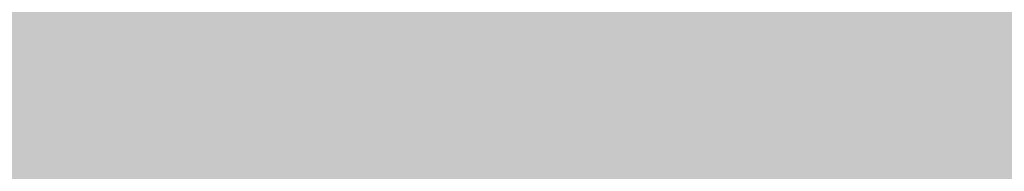
# Model space of a CAD drawing. Units: millimetres. Extents: x 0 to 2267, y 0 to 1823.
# Tile 48 of 256: x 1595.098 to 1596.855, y 1226.115 to 1226.386. Entities that reach past the tile are written whole.
import ezdxf

# ---------------------------------------------------------------- set-up
doc = ezdxf.new("R2010")
doc.units = ezdxf.units.MM
doc.header["$MEASUREMENT"] = 0
doc.layers.add('M-HATC', color=252, linetype='Continuous', lineweight=18)

msp = doc.modelspace()

# ---------------------------------------------------------------- hatches: boundary and pattern name
at = {"layer": 'M-HATC'}
h = msp.add_hatch(color=256, dxfattribs=at)
h.dxf.hatch_style = 1
h.paths.add_polyline_path([(2055.771, 1603.062), (1381.0868, 1603.062), (1381.0868, 1598.062), (2055.771, 1598.062)])
h.paths.add_polyline_path([(2055.771, 1598.062), (1381.0868, 1598.062), (1381.0868, 1593.062), (2055.771, 1593.062)])
h.paths.add_polyline_path([(2051.3074, 1536.7609), (1385.5504, 1536.7609), (1385.5504, 1526.7609), (1387.5504, 1526.7609), (1388.5366, 1525.0528), (1385.3319, 1521.2335), (1385.3319, 1521.2226), (2050.2542, 1522.7491), (2048.3212, 1525.0528), (2049.3074, 1526.7609), (2051.3074, 1526.7609)])
edge = h.paths.add_edge_path()
edge.add_arc((1847.5345, 1379.1492), 135, 222.603061, 222.890851, ccw=False)
edge.add_line((1748.1663, 1287.7656), (1683.0921, 1287.7656))
edge.add_arc((1583.7239, 1379.1492), 135, 317.109149, 317.396939, ccw=False)
edge.add_arc((1678.9686, 1290.6707), 5, 222.8909, 317.1091, ccw=False)
edge.add_arc((1774.2133, 1379.1492), 135, 222.603061, 222.890851, ccw=False)
edge.add_line((1674.8451, 1287.7656), (1609.7709, 1287.7656))
edge.add_arc((1510.4027, 1379.1492), 135, 317.109149, 317.396939, ccw=False)
edge.add_arc((1605.6474, 1290.6707), 5, 222.8909, 317.1091, ccw=False)
edge.add_arc((1700.8921, 1379.1492), 135, 222.603061, 222.890851, ccw=False)
edge.add_line((1601.5239, 1287.7656), (1536.4497, 1287.7656))
edge.add_arc((1437.0815, 1379.1492), 135, 317.109149, 317.396939, ccw=False)
edge.add_arc((1532.3262, 1290.6707), 5, 222.8909, 317.1091, ccw=False)
edge.add_arc((1627.5709, 1379.1492), 135, 222.603061, 222.890851, ccw=False)
edge.add_line((1528.2027, 1287.7656), (1505.9289, 1287.7656))
edge.add_spline(control_points=[(1505.9289, 1287.7656), (1504.2622, 1287.7656), (1504.2622, 1282.7656), (1505.9289, 1282.7656)], knot_values=[0, 0, 0, 0, 5, 5, 5, 5], degree=3, periodic=0)
edge.add_line((1505.9289, 1282.7656), (1930.9289, 1282.7656))
edge.add_spline(control_points=[(1930.9289, 1282.7656), (1932.5956, 1282.7656), (1932.5956, 1287.7656), (1930.9289, 1287.7656)], knot_values=[0, 0, 0, 0, 5, 5, 5, 5], degree=3, periodic=0)
edge.add_line((1930.9289, 1287.7656), (1903.0557, 1287.7656))
edge.add_arc((1803.6875, 1379.1492), 135, 317.109149, 317.396939, ccw=False)
edge.add_arc((1898.9322, 1290.6707), 5, 222.8909, 317.1091, ccw=False)
edge.add_arc((1994.1769, 1379.1492), 135, 222.603061, 222.890851, ccw=False)
edge.add_line((1894.8087, 1287.7656), (1829.7345, 1287.7656))
edge.add_arc((1730.3663, 1379.1492), 135, 317.109149, 317.396939, ccw=False)
edge.add_arc((1825.611, 1290.6707), 5, 222.8909, 317.1091, ccw=False)
edge.add_arc((1920.8557, 1379.1492), 135, 222.603061, 222.890851, ccw=False)
edge.add_line((1821.4875, 1287.7656), (1756.4133, 1287.7656))
edge.add_arc((1657.0451, 1379.1492), 135, 317.109149, 317.396939, ccw=False)
edge.add_arc((1752.2898, 1290.6707), 5, 222.8909, 317.1091, ccw=False)
edge = h.paths.add_edge_path()
edge.add_spline(control_points=[(1843.4289, 1227.2475), (1845.0956, 1227.2475), (1845.0956, 1232.2475), (1843.4289, 1232.2475)], knot_values=[0, 0, 0, 0, 5, 5, 5, 5], degree=3, periodic=0)
edge.add_line((1843.4289, 1232.2475), (1593.4289, 1232.2475))
edge.add_spline(control_points=[(1593.4289, 1232.2475), (1591.7622, 1232.2475), (1591.7622, 1227.2475), (1593.4289, 1227.2475)], knot_values=[0, 0, 0, 0, 5, 5, 5, 5], degree=3, periodic=0)
edge.add_line((1593.4289, 1227.2475), (1843.4289, 1227.2475))
h.paths.add_polyline_path([(1905.9289, 1127.4171), (1530.9289, 1127.4171, 0.414214), (1520.9289, 1117.4171), (1530.9289, 1117.4171), (1915.9289, 1117.4171, 0.414214)])
edge = h.paths.add_edge_path()
edge.add_arc((1397.0858, 1498.4078), 12.7299, 90.78215, 190.87871, ccw=False)
edge.add_line((1396.912, 1511.1365), (1428.0097, 1511.3488))
edge.add_line((1428.0097, 1511.3488), (1433.0097, 1511.3488))
edge.add_line((1433.0097, 1511.3488), (1434.439, 1511.3488))
edge.add_arc((1419.474, 1498.0804), 20, 41.561, 74.08211)
edge.add_line((1424.9592, 1517.3135), (1399.9351, 1517.2561))
edge.add_spline(control_points=[(1399.9307, 1517.2561), (1399.884, 1517.2131), (1399.8328, 1517.1689), (1399.7774, 1517.1236)], knot_values=[11.567499, 11.567499, 11.567499, 11.567499, 11.814249, 11.814249, 11.814249, 11.814249], degree=3, periodic=0)
edge.add_spline(control_points=[(1399.6328, 1517.0099), (1399.5831, 1516.9721), (1399.5307, 1516.9338), (1399.4759, 1516.8947)], knot_values=[11.167718, 11.167718, 11.167718, 11.167718, 11.365188, 11.365188, 11.365188, 11.365188], degree=3, periodic=0)
edge.add_spline(control_points=[(1399.3398, 1516.8001), (1399.1514, 1516.6719), (1398.9384, 1516.5377), (1398.704, 1516.3994)], knot_values=[10.376405, 10.376405, 10.376405, 10.376405, 11.00994, 11.00994, 11.00994, 11.00994], degree=3, periodic=0)
edge.add_spline(control_points=[(1398.6572, 1516.3719), (1398.5789, 1516.326), (1398.4983, 1516.2797), (1398.4155, 1516.2331)], knot_values=[10.125175, 10.125175, 10.125175, 10.125175, 10.334406, 10.334406, 10.334406, 10.334406], degree=3, periodic=0)
edge.add_spline(control_points=[(1398.2642, 1516.1487), (1398.196, 1516.1111), (1398.1263, 1516.0732), (1398.0555, 1516.0351)], knot_values=[9.832246, 9.832246, 9.832246, 9.832246, 9.999658, 9.999658, 9.999658, 9.999658], degree=3, periodic=0)
edge.add_spline(control_points=[(1397.9987, 1516.0048), (1397.7312, 1515.8621), (1397.446, 1515.7171), (1397.1466, 1515.5714)], knot_values=[9.161808, 9.161808, 9.161808, 9.161808, 9.787769, 9.787769, 9.787769, 9.787769], degree=3, periodic=0)
edge.add_spline(control_points=[(1397.1466, 1515.5714), (1396.8418, 1515.423), (1396.5222, 1515.274), (1396.1914, 1515.1262)], knot_values=[8.524455, 8.524455, 8.524455, 8.524455, 9.161808, 9.161808, 9.161808, 9.161808], degree=3, periodic=0)
edge.add_spline(control_points=[(1396.0777, 1515.0756), (1395.9854, 1515.0348), (1395.8922, 1514.994), (1395.7983, 1514.9534)], knot_values=[8.275193, 8.275193, 8.275193, 8.275193, 8.451726, 8.451726, 8.451726, 8.451726], degree=3, periodic=0)
edge.add_spline(control_points=[(1395.6018, 1514.8691), (1395.4997, 1514.8257), (1395.3968, 1514.7824), (1395.2932, 1514.7394)], knot_values=[7.962917, 7.962917, 7.962917, 7.962917, 8.152764, 8.152764, 8.152764, 8.152764], degree=3, periodic=0)
edge.add_spline(control_points=[(1395.2116, 1514.7057), (1394.8278, 1514.5475), (1394.4345, 1514.3929), (1394.0364, 1514.2442)], knot_values=[7.21254, 7.21254, 7.21254, 7.21254, 7.913148, 7.913148, 7.913148, 7.913148], degree=3, periodic=0)
edge.add_spline(control_points=[(1394.0364, 1514.2442), (1393.7076, 1514.1214), (1393.3754, 1514.0027), (1393.0427, 1513.8895)], knot_values=[6.633733, 6.633733, 6.633733, 6.633733, 7.21254, 7.21254, 7.21254, 7.21254], degree=3, periodic=0)
edge.add_spline(control_points=[(1392.8214, 1513.815), (1392.7198, 1513.7812), (1392.6181, 1513.7479), (1392.5166, 1513.7152)], knot_values=[6.328796, 6.328796, 6.328796, 6.328796, 6.505493, 6.505493, 6.505493, 6.505493], degree=3, periodic=0)
edge.add_spline(control_points=[(1392.5166, 1513.7152), (1392.3187, 1513.6515), (1392.1212, 1513.59), (1391.9244, 1513.531)], knot_values=[5.984605, 5.984605, 5.984605, 5.984605, 6.328796, 6.328796, 6.328796, 6.328796], degree=3, periodic=0)
edge.add_spline(control_points=[(1391.7915, 1513.4915), (1391.3122, 1513.3501), (1390.8384, 1513.2239), (1390.3784, 1513.1171)], knot_values=[5.066697, 5.066697, 5.066697, 5.066697, 5.907055, 5.907055, 5.907055, 5.907055], degree=3, periodic=0)
edge.add_spline(control_points=[(1390.3784, 1513.1171), (1390.1797, 1513.071), (1389.9836, 1513.0284), (1389.7907, 1512.9899)], knot_values=[4.70367, 4.70367, 4.70367, 4.70367, 5.066695, 5.066695, 5.066695, 5.066695], degree=3, periodic=0)
edge.add_spline(control_points=[(1389.422, 1512.9204), (1389.2459, 1512.8892), (1389.0729, 1512.8617), (1388.9036, 1512.8381)], knot_values=[4.130571, 4.130571, 4.130571, 4.130571, 4.469816, 4.469816, 4.469816, 4.469816], degree=3, periodic=0)
edge.add_spline(control_points=[(1388.9036, 1512.8381), (1388.591, 1512.7946), (1388.2911, 1512.7644), (1388.0071, 1512.7494)], knot_values=[3.504031, 3.504031, 3.504031, 3.504031, 4.130571, 4.130571, 4.130571, 4.130571], degree=3, periodic=0)
edge.add_spline(control_points=[(1387.9356, 1512.7459), (1387.8538, 1512.7423), (1387.7733, 1512.74), (1387.6944, 1512.739)], knot_values=[3.268866, 3.268866, 3.268866, 3.268866, 3.451164, 3.451164, 3.451164, 3.451164], degree=3, periodic=0)
edge.add_spline(control_points=[(1387.3351, 1512.7443), (1387.2076, 1512.7499), (1387.0847, 1512.7597), (1386.967, 1512.7739)], knot_values=[2.670686, 2.670686, 2.670686, 2.670686, 2.984, 2.984, 2.984, 2.984], degree=3, periodic=0)
edge.add_spline(control_points=[(1386.8327, 1512.7922), (1386.8209, 1512.7941), (1386.8092, 1512.7959), (1386.7975, 1512.7979)], knot_values=[2.516981, 2.516981, 2.516981, 2.516981, 2.549528, 2.549528, 2.549528, 2.549528], degree=3, periodic=0)
edge.add_spline(control_points=[(1386.4526, 1512.8735), (1386.4257, 1512.881), (1386.3993, 1512.889), (1386.3733, 1512.8972)], knot_values=[2.095869, 2.095869, 2.095869, 2.095869, 2.17941, 2.17941, 2.17941, 2.17941], degree=3, periodic=0)
edge.add_spline(control_points=[(1386.0691, 1513.0189), (1386.0634, 1513.0217), (1386.0577, 1513.0246), (1386.052, 1513.0275)], knot_values=[1.72453, 1.72453, 1.72453, 1.72453, 1.745933, 1.745933, 1.745933, 1.745933], degree=3, periodic=0)
edge.add_arc((1399.474, 1498.0804), 20, 131.82432, 180)
edge.add_arc((1630.3336, 1505.5484), 250.9708, 181.705176, 236.427975)
edge.add_arc((1605.3399, 1483.3044), 218.7822, 238.660829, 243.34961)
edge.add_arc((1647.0911, 1510.3592), 262.8986, 183.129836, 237.853442, ccw=False)
h.paths.add_polyline_path([(1406.5369, 1391.9644, 0.149382), (1491.5506, 1296.4418, -0.129517)], flags=17)
edge = h.paths.add_edge_path()
edge.add_arc((2037.3838, 1498.0804), 20, 0, 48.26587)
edge.add_spline(control_points=[(2050.6973, 1513.0052), (2050.6512, 1512.9847), (2050.6034, 1512.9655), (2050.5539, 1512.9477)], knot_values=[1.835652, 1.835652, 1.835652, 1.835652, 2.000781, 2.000781, 2.000781, 2.000781], degree=3, periodic=0)
edge.add_spline(control_points=[(2050.4616, 1512.9166), (2050.479, 1512.9221), (2050.4963, 1512.9277), (2050.5133, 1512.9335)], knot_values=[2.045477, 2.045477, 2.045477, 2.045477, 2.101389, 2.101389, 2.101389, 2.101389], degree=3, periodic=0)
edge.add_spline(control_points=[(2050.129, 1512.8342), (2050.1984, 1512.8473), (2050.2657, 1512.8623), (2050.3308, 1512.8792)], knot_values=[2.237629, 2.237629, 2.237629, 2.237629, 2.435841, 2.435841, 2.435841, 2.435841], degree=3, periodic=0)
edge.add_spline(control_points=[(2050.0946, 1512.8278), (2050.1061, 1512.8299), (2050.1176, 1512.832), (2050.129, 1512.8342)], knot_values=[2.435841, 2.435841, 2.435841, 2.435841, 2.468321, 2.468321, 2.468321, 2.468321], degree=3, periodic=0)
edge.add_spline(control_points=[(2049.7843, 1512.7851), (2049.8552, 1512.7922), (2049.9243, 1512.8008), (2049.9917, 1512.8109)], knot_values=[2.563852, 2.563852, 2.563852, 2.563852, 2.748541, 2.748541, 2.748541, 2.748541], degree=3, periodic=0)
edge.add_spline(control_points=[(2049.4052, 1512.7617), (2049.5364, 1512.7653), (2049.6629, 1512.773), (2049.7843, 1512.7851)], knot_values=[2.748541, 2.748541, 2.748541, 2.748541, 3.064882, 3.064882, 3.064882, 3.064882], degree=3, periodic=0)
edge.add_spline(control_points=[(2049.1698, 1512.7597), (2049.2336, 1512.7591), (2049.2965, 1512.7594), (2049.3584, 1512.7606)], knot_values=[3.102309, 3.102309, 3.102309, 3.102309, 3.2503, 3.2503, 3.2503, 3.2503], degree=3, periodic=0)
edge.add_spline(control_points=[(2048.8573, 1512.7691), (2048.9638, 1512.7638), (2049.068, 1512.7606), (2049.1698, 1512.7597)], knot_values=[3.2503, 3.2503, 3.2503, 3.2503, 3.486069, 3.486069, 3.486069, 3.486069], degree=3, periodic=0)
edge.add_spline(control_points=[(2048.6924, 1512.7789), (2048.3729, 1512.8009), (2048.0345, 1512.8411), (2047.6817, 1512.897)], knot_values=[3.606429, 3.606429, 3.606429, 3.606429, 4.2989, 4.2989, 4.2989, 4.2989], degree=3, periodic=0)
edge.add_spline(control_points=[(2047.6817, 1512.897), (2047.5458, 1512.9185), (2047.4077, 1512.9424), (2047.2678, 1512.9685)], knot_values=[4.2989, 4.2989, 4.2989, 4.2989, 4.565769, 4.565769, 4.565769, 4.565769], degree=3, periodic=0)
edge.add_spline(control_points=[(2047.2678, 1512.9685), (2047.1449, 1512.9914), (2047.0207, 1513.016), (2046.8951, 1513.0422)], knot_values=[4.565769, 4.565769, 4.565769, 4.565769, 4.799971, 4.799971, 4.799971, 4.799971], degree=3, periodic=0)
edge.add_spline(control_points=[(2046.8951, 1513.0422), (2046.5286, 1513.1188), (2046.1513, 1513.209), (2045.7676, 1513.3107)], knot_values=[4.799971, 4.799971, 4.799971, 4.799971, 5.483718, 5.483718, 5.483718, 5.483718], degree=3, periodic=0)
edge.add_spline(control_points=[(2045.7676, 1513.3107), (2045.3724, 1513.4154), (2044.9704, 1513.5322), (2044.5662, 1513.6588)], knot_values=[5.483718, 5.483718, 5.483718, 5.483718, 6.187866, 6.187866, 6.187866, 6.187866], degree=3, periodic=0)
edge.add_spline(control_points=[(2044.5662, 1513.6588), (2044.4149, 1513.7061), (2044.2633, 1513.7549), (2044.1116, 1513.8048)], knot_values=[6.187866, 6.187866, 6.187866, 6.187866, 6.451551, 6.451551, 6.451551, 6.451551], degree=3, periodic=0)
edge.add_spline(control_points=[(2044.1116, 1513.8048), (2043.9967, 1513.8427), (2043.8817, 1513.8813), (2043.7668, 1513.9205)], knot_values=[6.451551, 6.451551, 6.451551, 6.451551, 6.651434, 6.651434, 6.651434, 6.651434], degree=3, periodic=0)
edge.add_spline(control_points=[(2043.7668, 1513.9205), (2043.3716, 1514.0554), (2042.9774, 1514.1979), (2042.5886, 1514.3458)], knot_values=[6.651434, 6.651434, 6.651434, 6.651434, 7.338879, 7.338879, 7.338879, 7.338879], degree=3, periodic=0)
edge.add_spline(control_points=[(2042.5886, 1514.3458), (2042.1643, 1514.5071), (2041.7465, 1514.6749), (2041.3409, 1514.846)], knot_values=[7.338879, 7.338879, 7.338879, 7.338879, 8.089209, 8.089209, 8.089209, 8.089209], degree=3, periodic=0)
edge.add_spline(control_points=[(2041.3409, 1514.846), (2041.1028, 1514.9465), (2040.869, 1515.0481), (2040.6405, 1515.1502)], knot_values=[8.089209, 8.089209, 8.089209, 8.089209, 8.529587, 8.529587, 8.529587, 8.529587], degree=3, periodic=0)
edge.add_spline(control_points=[(2040.51, 1515.2089), (2040.0824, 1515.4022), (2039.6747, 1515.5971), (2039.295, 1515.7894)], knot_values=[8.613818, 8.613818, 8.613818, 8.613818, 9.44571, 9.44571, 9.44571, 9.44571], degree=3, periodic=0)
edge.add_spline(control_points=[(2039.295, 1515.7894), (2039.0618, 1515.9075), (2038.8391, 1516.0246), (2038.6288, 1516.1398)], knot_values=[9.44571, 9.44571, 9.44571, 9.44571, 9.956404, 9.956404, 9.956404, 9.956404], degree=3, periodic=0)
edge.add_spline(control_points=[(2038.6288, 1516.1398), (2038.5187, 1516.2001), (2038.4121, 1516.2598), (2038.309, 1516.3189)], knot_values=[9.956404, 9.956404, 9.956404, 9.956404, 10.223542, 10.223542, 10.223542, 10.223542], degree=3, periodic=0)
edge.add_spline(control_points=[(2038.309, 1516.3189), (2038.2138, 1516.3735), (2038.1216, 1516.4276), (2038.0328, 1516.481)], knot_values=[10.223542, 10.223542, 10.223542, 10.223542, 10.47051, 10.47051, 10.47051, 10.47051], degree=3, periodic=0)
edge.add_spline(control_points=[(2038.0328, 1516.481), (2037.7855, 1516.6296), (2037.5639, 1516.773), (2037.3722, 1516.909)], knot_values=[10.47051, 10.47051, 10.47051, 10.47051, 11.15767, 11.15767, 11.15767, 11.15767], degree=3, periodic=0)
edge.add_spline(control_points=[(2037.3722, 1516.909), (2037.2789, 1516.9752), (2037.1927, 1517.0396), (2037.1142, 1517.102)], knot_values=[11.15767, 11.15767, 11.15767, 11.15767, 11.49227, 11.49227, 11.49227, 11.49227], degree=3, periodic=0)
edge.add_spline(control_points=[(2036.8564, 1517.3259), (2036.9148, 1517.2692), (2036.9814, 1517.2103), (2037.0557, 1517.1492)], knot_values=[11.577341, 11.577341, 11.577341, 11.577341, 11.91035, 11.91035, 11.91035, 11.91035], degree=3, periodic=0)
edge.add_spline(control_points=[(2036.8074, 1517.3748), (2036.823, 1517.3587), (2036.8393, 1517.3424), (2036.8564, 1517.3259)], knot_values=[11.91035, 11.91035, 11.91035, 11.91035, 12.007402, 12.007402, 12.007402, 12.007402], degree=3, periodic=0)
edge.add_spline(control_points=[(2036.7017, 1517.494), (2036.7104, 1517.483), (2036.7196, 1517.4719), (2036.7291, 1517.4606)], knot_values=[12.184155, 12.184155, 12.184155, 12.184155, 12.255409, 12.255409, 12.255409, 12.255409], degree=3, periodic=0)
edge.add_spline(control_points=[(2036.6159, 1517.6205), (2036.62, 1517.613), (2036.6243, 1517.6055), (2036.6289, 1517.5979)], knot_values=[12.487913, 12.487913, 12.487913, 12.487913, 12.541035, 12.541035, 12.541035, 12.541035], degree=3, periodic=0)
edge.add_spline(control_points=[(2036.5635, 1517.786), (2036.5637, 1517.7794), (2036.5642, 1517.7726), (2036.565, 1517.7658)], knot_values=[12.911761, 12.911761, 12.911761, 12.911761, 12.968286, 12.968286, 12.968286, 12.968286], degree=3, periodic=0)
edge.add_spline(control_points=[(2036.6166, 1517.9304), (2036.6125, 1517.9259), (2036.6086, 1517.9212), (2036.6049, 1517.9165)], knot_values=[13.382527, 13.382527, 13.382527, 13.382527, 13.433791, 13.433791, 13.433791, 13.433791], degree=3, periodic=0)
edge.add_spline(control_points=[(2036.749, 1518.017), (2036.7361, 1518.0116), (2036.7239, 1518.006), (2036.7124, 1518.0002)], knot_values=[13.726299, 13.726299, 13.726299, 13.726299, 13.809928, 13.809928, 13.809928, 13.809928], degree=3, periodic=0)
edge.add_spline(control_points=[(2036.8604, 1518.0528), (2036.8386, 1518.0474), (2036.8181, 1518.0416), (2036.7988, 1518.0353)], knot_values=[13.910887, 13.910887, 13.910887, 13.910887, 14.02153, 14.02153, 14.02153, 14.02153], degree=3, periodic=0)
edge.add_line((2036.9639, 1518.0804), (2032.3838, 1518.0804))
edge.add_line((2032.3838, 1518.0804), (2027.3838, 1518.0804))
edge.add_line((2027.3838, 1518.0804), (2022.3838, 1518.0804))
edge.add_line((2022.3838, 1518.0804), (2017.3838, 1518.0804))
edge.add_arc((2017.3838, 1498.0804), 20, 90, 138.439)
edge.add_line((2002.4188, 1511.3488), (2003.8481, 1511.3488))
edge.add_line((2003.8481, 1511.3488), (2008.8481, 1511.3488))
edge.add_line((2008.8481, 1511.3488), (2039.772, 1511.1377))
edge.add_arc((2039.772, 1498.4078), 12.7299, -10.87871, 90, ccw=False)
edge.add_arc((1789.7668, 1510.3592), 262.8986, 302.146558, 356.870164, ccw=False)
edge.add_arc((1831.5179, 1483.3044), 218.7822, 296.65039, 301.339171)
edge.add_arc((1806.5242, 1505.5484), 250.9708, 303.572025, 358.294824)
h.paths.add_polyline_path([(2030.321, 1391.9644, -0.129517), (1945.3072, 1296.4418, 0.149382)], flags=17)
edge = h.paths.add_edge_path()
edge.add_spline(control_points=[(2037.2464, 1518.0821), (2037.2898, 1518.081), (2037.3355, 1518.0804), (2037.3838, 1518.0804)], knot_values=[0.000012, 0.000012, 0.000012, 0.000012, 0.144754, 0.144754, 0.144754, 0.144754], degree=3, periodic=0)
edge.add_line((2037.3357, 1518.0804), (2037.0096, 1518.0804))
edge.add_spline(control_points=[(2037.0096, 1518.0804), (2036.9822, 1518.0768), (2036.956, 1518.0727), (2036.9312, 1518.0681)], knot_values=[14.13465, 14.13465, 14.13465, 14.13465, 14.247197, 14.247197, 14.247197, 14.247197], degree=3, periodic=0)
edge.add_spline(control_points=[(2036.9312, 1518.0681), (2036.9276, 1518.0674), (2036.9241, 1518.0667), (2036.9205, 1518.0661)], knot_values=[14.118315, 14.118315, 14.118315, 14.118315, 14.13465, 14.13465, 14.13465, 14.13465], degree=3, periodic=0)
edge.add_spline(control_points=[(2036.9205, 1518.0661), (2036.9118, 1518.0644), (2036.9032, 1518.0626), (2036.8948, 1518.0608)], knot_values=[14.078086, 14.078086, 14.078086, 14.078086, 14.118315, 14.118315, 14.118315, 14.118315], degree=3, periodic=0)
edge.add_spline(control_points=[(2036.8948, 1518.0608), (2036.883, 1518.0583), (2036.8716, 1518.0556), (2036.8604, 1518.0528)], knot_values=[14.02153, 14.02153, 14.02153, 14.02153, 14.078086, 14.078086, 14.078086, 14.078086], degree=3, periodic=0)
edge.add_spline(control_points=[(2036.8604, 1518.0528), (2036.8386, 1518.0474), (2036.8181, 1518.0416), (2036.7988, 1518.0353)], knot_values=[13.910887, 13.910887, 13.910887, 13.910887, 14.02153, 14.02153, 14.02153, 14.02153], degree=3, periodic=0)
edge.add_spline(control_points=[(2036.7988, 1518.0353), (2036.7981, 1518.035), (2036.7974, 1518.0348), (2036.7967, 1518.0346)], knot_values=[13.906906, 13.906906, 13.906906, 13.906906, 13.910887, 13.910887, 13.910887, 13.910887], degree=3, periodic=0)
edge.add_spline(control_points=[(2036.7967, 1518.0346), (2036.7882, 1518.0318), (2036.7799, 1518.0289), (2036.7719, 1518.0259)], knot_values=[13.857826, 13.857826, 13.857826, 13.857826, 13.906906, 13.906906, 13.906906, 13.906906], degree=3, periodic=0)
edge.add_spline(control_points=[(2036.7719, 1518.0259), (2036.764, 1518.023), (2036.7564, 1518.02), (2036.749, 1518.017)], knot_values=[13.809928, 13.809928, 13.809928, 13.809928, 13.857826, 13.857826, 13.857826, 13.857826], degree=3, periodic=0)
edge.add_spline(control_points=[(2036.749, 1518.017), (2036.7361, 1518.0116), (2036.7239, 1518.006), (2036.7124, 1518.0002)], knot_values=[13.726299, 13.726299, 13.726299, 13.726299, 13.809928, 13.809928, 13.809928, 13.809928], degree=3, periodic=0)
edge.add_spline(control_points=[(2036.7124, 1518.0002), (2036.7121, 1518), (2036.7118, 1517.9999), (2036.7115, 1517.9997)], knot_values=[13.723993, 13.723993, 13.723993, 13.723993, 13.726299, 13.726299, 13.726299, 13.726299], degree=3, periodic=0)
edge.add_spline(control_points=[(2036.7115, 1517.9997), (2036.7063, 1517.9971), (2036.7013, 1517.9944), (2036.6965, 1517.9917)], knot_values=[13.686536, 13.686536, 13.686536, 13.686536, 13.723993, 13.723993, 13.723993, 13.723993], degree=3, periodic=0)
edge.add_spline(control_points=[(2036.6965, 1517.9917), (2036.6919, 1517.9891), (2036.6874, 1517.9865), (2036.6831, 1517.9839)], knot_values=[13.651251, 13.651251, 13.651251, 13.651251, 13.686536, 13.686536, 13.686536, 13.686536], degree=3, periodic=0)
edge.add_spline(control_points=[(2036.6831, 1517.9839), (2036.6764, 1517.9798), (2036.67, 1517.9757), (2036.6639, 1517.9714)], knot_values=[13.596804, 13.596804, 13.596804, 13.596804, 13.651251, 13.651251, 13.651251, 13.651251], degree=3, periodic=0)
edge.add_spline(control_points=[(2036.6639, 1517.9714), (2036.6636, 1517.9712), (2036.6633, 1517.9709), (2036.6629, 1517.9707)], knot_values=[13.593956, 13.593956, 13.593956, 13.593956, 13.596804, 13.596804, 13.596804, 13.596804], degree=3, periodic=0)
edge.add_spline(control_points=[(2036.6629, 1517.9707), (2036.6603, 1517.9689), (2036.6577, 1517.967), (2036.6552, 1517.9651)], knot_values=[13.570322, 13.570322, 13.570322, 13.570322, 13.593956, 13.593956, 13.593956, 13.593956], degree=3, periodic=0)
edge.add_spline(control_points=[(2036.6552, 1517.9651), (2036.6525, 1517.9631), (2036.6499, 1517.9611), (2036.6474, 1517.9591)], knot_values=[13.545477, 13.545477, 13.545477, 13.545477, 13.570322, 13.570322, 13.570322, 13.570322], degree=3, periodic=0)
edge.add_spline(control_points=[(2036.6474, 1517.9591), (2036.6472, 1517.9589), (2036.6471, 1517.9588), (2036.6469, 1517.9587)], knot_values=[13.543931, 13.543931, 13.543931, 13.543931, 13.545477, 13.545477, 13.545477, 13.545477], degree=3, periodic=0)
edge.add_spline(control_points=[(2036.6469, 1517.9587), (2036.6412, 1517.9541), (2036.6358, 1517.9494), (2036.6307, 1517.9447)], knot_values=[13.488237, 13.488237, 13.488237, 13.488237, 13.543931, 13.543931, 13.543931, 13.543931], degree=3, periodic=0)
edge.add_spline(control_points=[(2036.6307, 1517.9447), (2036.6282, 1517.9423), (2036.6257, 1517.9399), (2036.6233, 1517.9374)], knot_values=[13.460307, 13.460307, 13.460307, 13.460307, 13.488237, 13.488237, 13.488237, 13.488237], degree=3, periodic=0)
edge.add_spline(control_points=[(2036.6233, 1517.9374), (2036.6215, 1517.9356), (2036.6198, 1517.9338), (2036.6181, 1517.932)], knot_values=[13.439712, 13.439712, 13.439712, 13.439712, 13.460307, 13.460307, 13.460307, 13.460307], degree=3, periodic=0)
edge.add_spline(control_points=[(2036.6181, 1517.932), (2036.6176, 1517.9315), (2036.6171, 1517.9309), (2036.6166, 1517.9304)], knot_values=[13.433791, 13.433791, 13.433791, 13.433791, 13.439712, 13.439712, 13.439712, 13.439712], degree=3, periodic=0)
edge.add_spline(control_points=[(2036.6166, 1517.9304), (2036.6125, 1517.9259), (2036.6086, 1517.9212), (2036.6049, 1517.9165)], knot_values=[13.382527, 13.382527, 13.382527, 13.382527, 13.433791, 13.433791, 13.433791, 13.433791], degree=3, periodic=0)
edge.add_spline(control_points=[(2036.6049, 1517.9165), (2036.6026, 1517.9135), (2036.6004, 1517.9104), (2036.5982, 1517.9074)], knot_values=[13.350017, 13.350017, 13.350017, 13.350017, 13.382527, 13.382527, 13.382527, 13.382527], degree=3, periodic=0)
edge.add_spline(control_points=[(2036.5982, 1517.9074), (2036.5972, 1517.9059), (2036.5962, 1517.9043), (2036.5952, 1517.9028)], knot_values=[13.333922, 13.333922, 13.333922, 13.333922, 13.350017, 13.350017, 13.350017, 13.350017], degree=3, periodic=0)
edge.add_spline(control_points=[(2036.5952, 1517.9028), (2036.5945, 1517.9018), (2036.5939, 1517.9009), (2036.5933, 1517.8999)], knot_values=[13.323828, 13.323828, 13.323828, 13.323828, 13.333922, 13.333922, 13.333922, 13.333922], degree=3, periodic=0)
edge.add_spline(control_points=[(2036.5933, 1517.8999), (2036.5905, 1517.8955), (2036.5879, 1517.8909), (2036.5855, 1517.8864)], knot_values=[13.277545, 13.277545, 13.277545, 13.277545, 13.323828, 13.323828, 13.323828, 13.323828], degree=3, periodic=0)
edge.add_spline(control_points=[(2036.5855, 1517.8864), (2036.5836, 1517.8827), (2036.5817, 1517.8789), (2036.5801, 1517.8751)], knot_values=[13.240119, 13.240119, 13.240119, 13.240119, 13.277545, 13.277545, 13.277545, 13.277545], degree=3, periodic=0)
edge.add_spline(control_points=[(2036.5801, 1517.8751), (2036.5795, 1517.8739), (2036.579, 1517.8727), (2036.5785, 1517.8715)], knot_values=[13.228211, 13.228211, 13.228211, 13.228211, 13.240119, 13.240119, 13.240119, 13.240119], degree=3, periodic=0)
edge.add_spline(control_points=[(2036.5785, 1517.8715), (2036.578, 1517.8702), (2036.5774, 1517.869), (2036.5769, 1517.8677)], knot_values=[13.215717, 13.215717, 13.215717, 13.215717, 13.228211, 13.228211, 13.228211, 13.228211], degree=3, periodic=0)
edge.add_spline(control_points=[(2036.5769, 1517.8677), (2036.5755, 1517.864), (2036.5741, 1517.8603), (2036.5729, 1517.8565)], knot_values=[13.179847, 13.179847, 13.179847, 13.179847, 13.215717, 13.215717, 13.215717, 13.215717], degree=3, periodic=0)
edge.add_spline(control_points=[(2036.5729, 1517.8565), (2036.5713, 1517.8515), (2036.5699, 1517.8464), (2036.5687, 1517.8413)], knot_values=[13.132017, 13.132017, 13.132017, 13.132017, 13.179847, 13.179847, 13.179847, 13.179847], degree=3, periodic=0)
edge.add_spline(control_points=[(2036.5687, 1517.8413), (2036.5684, 1517.8402), (2036.5682, 1517.8392), (2036.568, 1517.8382)], knot_values=[13.122482, 13.122482, 13.122482, 13.122482, 13.132017, 13.132017, 13.132017, 13.132017], degree=3, periodic=0)
edge.add_spline(control_points=[(2036.568, 1517.8382), (2036.5676, 1517.8363), (2036.5672, 1517.8345), (2036.5669, 1517.8327)], knot_values=[13.105592, 13.105592, 13.105592, 13.105592, 13.122482, 13.122482, 13.122482, 13.122482], degree=3, periodic=0)
edge.add_spline(control_points=[(2036.5669, 1517.8327), (2036.5662, 1517.8292), (2036.5657, 1517.8257), (2036.5652, 1517.8222)], knot_values=[13.074063, 13.074063, 13.074063, 13.074063, 13.105592, 13.105592, 13.105592, 13.105592], degree=3, periodic=0)
edge.add_spline(control_points=[(2036.5652, 1517.8222), (2036.5652, 1517.8222), (2036.5652, 1517.8222), (2036.5652, 1517.8222)], knot_values=[13.074043, 13.074043, 13.074043, 13.074043, 13.074063, 13.074063, 13.074063, 13.074063], degree=3, periodic=0)
edge.add_spline(control_points=[(2036.5652, 1517.8222), (2036.5644, 1517.8164), (2036.5639, 1517.8106), (2036.5636, 1517.8046)], knot_values=[13.021884, 13.021884, 13.021884, 13.021884, 13.074043, 13.074043, 13.074043, 13.074043], degree=3, periodic=0)
edge.add_spline(control_points=[(2036.5636, 1517.8046), (2036.5636, 1517.804), (2036.5636, 1517.8034), (2036.5635, 1517.8028)], knot_values=[13.01674, 13.01674, 13.01674, 13.01674, 13.021884, 13.021884, 13.021884, 13.021884], degree=3, periodic=0)
edge.add_spline(control_points=[(2036.5635, 1517.8028), (2036.5634, 1517.8005), (2036.5634, 1517.7982), (2036.5634, 1517.7958)], knot_values=[12.996438, 12.996438, 12.996438, 12.996438, 13.01674, 13.01674, 13.01674, 13.01674], degree=3, periodic=0)
edge.add_spline(control_points=[(2036.5634, 1517.7958), (2036.5633, 1517.7926), (2036.5634, 1517.7893), (2036.5635, 1517.786)], knot_values=[12.968286, 12.968286, 12.968286, 12.968286, 12.996438, 12.996438, 12.996438, 12.996438], degree=3, periodic=0)
edge.add_spline(control_points=[(2036.5635, 1517.786), (2036.5637, 1517.7794), (2036.5642, 1517.7726), (2036.565, 1517.7658)], knot_values=[12.911761, 12.911761, 12.911761, 12.911761, 12.968286, 12.968286, 12.968286, 12.968286], degree=3, periodic=0)
edge.add_spline(control_points=[(2036.565, 1517.7658), (2036.565, 1517.7657), (2036.565, 1517.7656), (2036.565, 1517.7656)], knot_values=[12.911017, 12.911017, 12.911017, 12.911017, 12.911761, 12.911761, 12.911761, 12.911761], degree=3, periodic=0)
edge.add_spline(control_points=[(2036.565, 1517.7656), (2036.5654, 1517.7625), (2036.5658, 1517.7593), (2036.5663, 1517.7562)], knot_values=[12.88528, 12.88528, 12.88528, 12.88528, 12.911017, 12.911017, 12.911017, 12.911017], degree=3, periodic=0)
edge.add_spline(control_points=[(2036.5663, 1517.7562), (2036.5667, 1517.7534), (2036.5672, 1517.7506), (2036.5677, 1517.7478)], knot_values=[12.862519, 12.862519, 12.862519, 12.862519, 12.88528, 12.88528, 12.88528, 12.88528], degree=3, periodic=0)
edge.add_spline(control_points=[(2036.5677, 1517.7478), (2036.5678, 1517.7474), (2036.5679, 1517.7469), (2036.568, 1517.7465)], knot_values=[12.858885, 12.858885, 12.858885, 12.858885, 12.862519, 12.862519, 12.862519, 12.862519], degree=3, periodic=0)
edge.add_spline(control_points=[(2036.568, 1517.7465), (2036.5692, 1517.7399), (2036.5707, 1517.7332), (2036.5724, 1517.7264)], knot_values=[12.8053, 12.8053, 12.8053, 12.8053, 12.858885, 12.858885, 12.858885, 12.858885], degree=3, periodic=0)
edge.add_spline(control_points=[(2036.5724, 1517.7264), (2036.5734, 1517.7226), (2036.5745, 1517.7187), (2036.5756, 1517.7149)], knot_values=[12.775176, 12.775176, 12.775176, 12.775176, 12.8053, 12.8053, 12.8053, 12.8053], degree=3, periodic=0)
edge.add_spline(control_points=[(2036.5756, 1517.7149), (2036.5763, 1517.7125), (2036.577, 1517.7102), (2036.5778, 1517.7078)], knot_values=[12.756759, 12.756759, 12.756759, 12.756759, 12.775176, 12.775176, 12.775176, 12.775176], degree=3, periodic=0)
edge.add_spline(control_points=[(2036.5778, 1517.7078), (2036.5781, 1517.7067), (2036.5784, 1517.7057), (2036.5787, 1517.7047)], knot_values=[12.748742, 12.748742, 12.748742, 12.748742, 12.756759, 12.756759, 12.756759, 12.756759], degree=3, periodic=0)
edge.add_spline(control_points=[(2036.5787, 1517.7047), (2036.5808, 1517.6983), (2036.5831, 1517.6919), (2036.5856, 1517.6854)], knot_values=[12.69959, 12.69959, 12.69959, 12.69959, 12.748742, 12.748742, 12.748742, 12.748742], degree=3, periodic=0)
edge.add_spline(control_points=[(2036.5856, 1517.6854), (2036.5876, 1517.68), (2036.5898, 1517.6746), (2036.5921, 1517.6692)], knot_values=[12.659038, 12.659038, 12.659038, 12.659038, 12.69959, 12.69959, 12.69959, 12.69959], degree=3, periodic=0)
edge.add_spline(control_points=[(2036.5921, 1517.6692), (2036.594, 1517.6648), (2036.5959, 1517.6605), (2036.5979, 1517.6561)], knot_values=[12.626806, 12.626806, 12.626806, 12.626806, 12.659038, 12.659038, 12.659038, 12.659038], degree=3, periodic=0)
edge.add_spline(control_points=[(2036.5979, 1517.6561), (2036.5984, 1517.6551), (2036.5989, 1517.6541), (2036.5993, 1517.6531)], knot_values=[12.619394, 12.619394, 12.619394, 12.619394, 12.626806, 12.626806, 12.626806, 12.626806], degree=3, periodic=0)
edge.add_spline(control_points=[(2036.5993, 1517.6531), (2036.6043, 1517.6424), (2036.6099, 1517.6315), (2036.6159, 1517.6205)], knot_values=[12.541039, 12.541039, 12.541039, 12.541039, 12.619394, 12.619394, 12.619394, 12.619394], degree=3, periodic=0)
edge.add_spline(control_points=[(2036.6159, 1517.6205), (2036.6159, 1517.6205), (2036.6159, 1517.6205), (2036.6159, 1517.6205)], knot_values=[12.541035, 12.541035, 12.541035, 12.541035, 12.541039, 12.541039, 12.541039, 12.541039], degree=3, periodic=0)
edge.add_spline(control_points=[(2036.6159, 1517.6205), (2036.62, 1517.613), (2036.6243, 1517.6055), (2036.6289, 1517.5979)], knot_values=[12.487913, 12.487913, 12.487913, 12.487913, 12.541035, 12.541035, 12.541035, 12.541035], degree=3, periodic=0)
edge.add_spline(control_points=[(2036.6289, 1517.5979), (2036.6326, 1517.5916), (2036.6365, 1517.5853), (2036.6406, 1517.5789)], knot_values=[12.443982, 12.443982, 12.443982, 12.443982, 12.487913, 12.487913, 12.487913, 12.487913], degree=3, periodic=0)
edge.add_spline(control_points=[(2036.6406, 1517.5789), (2036.6414, 1517.5776), (2036.6423, 1517.5763), (2036.6431, 1517.5749)], knot_values=[12.434996, 12.434996, 12.434996, 12.434996, 12.443982, 12.443982, 12.443982, 12.443982], degree=3, periodic=0)
edge.add_spline(control_points=[(2036.6431, 1517.5749), (2036.6531, 1517.5596), (2036.6639, 1517.5439), (2036.6756, 1517.528)], knot_values=[12.329647, 12.329647, 12.329647, 12.329647, 12.434996, 12.434996, 12.434996, 12.434996], degree=3, periodic=0)
edge.add_spline(control_points=[(2036.6756, 1517.528), (2036.6839, 1517.5168), (2036.6925, 1517.5055), (2036.7017, 1517.494)], knot_values=[12.255409, 12.255409, 12.255409, 12.255409, 12.329647, 12.329647, 12.329647, 12.329647], degree=3, periodic=0)
edge.add_spline(control_points=[(2036.7017, 1517.494), (2036.7104, 1517.483), (2036.7196, 1517.4719), (2036.7291, 1517.4606)], knot_values=[12.184155, 12.184155, 12.184155, 12.184155, 12.255409, 12.255409, 12.255409, 12.255409], degree=3, periodic=0)
edge.add_spline(control_points=[(2036.7291, 1517.4606), (2036.7436, 1517.4435), (2036.759, 1517.4262), (2036.7753, 1517.4085)], knot_values=[12.075961, 12.075961, 12.075961, 12.075961, 12.184155, 12.184155, 12.184155, 12.184155], degree=3, periodic=0)
edge.add_spline(control_points=[(2036.7753, 1517.4085), (2036.7763, 1517.4075), (2036.7773, 1517.4064), (2036.7783, 1517.4054)], knot_values=[12.069502, 12.069502, 12.069502, 12.069502, 12.075961, 12.075961, 12.075961, 12.075961], degree=3, periodic=0)
edge.add_spline(control_points=[(2036.7783, 1517.4054), (2036.7877, 1517.3953), (2036.7974, 1517.385), (2036.8074, 1517.3748)], knot_values=[12.007402, 12.007402, 12.007402, 12.007402, 12.069502, 12.069502, 12.069502, 12.069502], degree=3, periodic=0)
edge.add_spline(control_points=[(2036.8074, 1517.3748), (2036.823, 1517.3587), (2036.8393, 1517.3424), (2036.8564, 1517.3259)], knot_values=[11.91035, 11.91035, 11.91035, 11.91035, 12.007402, 12.007402, 12.007402, 12.007402], degree=3, periodic=0)
edge.add_spline(control_points=[(2036.8564, 1517.3259), (2036.9148, 1517.2692), (2036.9814, 1517.2103), (2037.0557, 1517.1492)], knot_values=[11.577341, 11.577341, 11.577341, 11.577341, 11.91035, 11.91035, 11.91035, 11.91035], degree=3, periodic=0)
edge.add_spline(control_points=[(2037.0557, 1517.1492), (2037.0747, 1517.1336), (2037.0942, 1517.1179), (2037.1142, 1517.102)], knot_values=[11.49227, 11.49227, 11.49227, 11.49227, 11.577341, 11.577341, 11.577341, 11.577341], degree=3, periodic=0)
edge.add_spline(control_points=[(2037.1142, 1517.102), (2037.1927, 1517.0396), (2037.2789, 1516.9752), (2037.3722, 1516.909)], knot_values=[11.15767, 11.15767, 11.15767, 11.15767, 11.49227, 11.49227, 11.49227, 11.49227], degree=3, periodic=0)
edge.add_spline(control_points=[(2037.3722, 1516.909), (2037.5639, 1516.773), (2037.7855, 1516.6296), (2038.0328, 1516.481)], knot_values=[10.47051, 10.47051, 10.47051, 10.47051, 11.15767, 11.15767, 11.15767, 11.15767], degree=3, periodic=0)
edge.add_spline(control_points=[(2038.0328, 1516.481), (2038.1216, 1516.4276), (2038.2138, 1516.3735), (2038.309, 1516.3189)], knot_values=[10.223542, 10.223542, 10.223542, 10.223542, 10.47051, 10.47051, 10.47051, 10.47051], degree=3, periodic=0)
edge.add_spline(control_points=[(2038.309, 1516.3189), (2038.4121, 1516.2598), (2038.5187, 1516.2001), (2038.6288, 1516.1398)], knot_values=[9.956404, 9.956404, 9.956404, 9.956404, 10.223542, 10.223542, 10.223542, 10.223542], degree=3, periodic=0)
edge.add_spline(control_points=[(2038.6288, 1516.1398), (2038.8391, 1516.0246), (2039.0618, 1515.9075), (2039.295, 1515.7894)], knot_values=[9.44571, 9.44571, 9.44571, 9.44571, 9.956404, 9.956404, 9.956404, 9.956404], degree=3, periodic=0)
edge.add_spline(control_points=[(2039.295, 1515.7894), (2039.6747, 1515.5971), (2040.0824, 1515.4022), (2040.51, 1515.2089)], knot_values=[8.613818, 8.613818, 8.613818, 8.613818, 9.44571, 9.44571, 9.44571, 9.44571], degree=3, periodic=0)
edge.add_spline(control_points=[(2040.51, 1515.2089), (2040.5533, 1515.1893), (2040.5968, 1515.1697), (2040.6405, 1515.1502)], knot_values=[8.529587, 8.529587, 8.529587, 8.529587, 8.613818, 8.613818, 8.613818, 8.613818], degree=3, periodic=0)
edge.add_spline(control_points=[(2040.6405, 1515.1502), (2040.869, 1515.0481), (2041.1028, 1514.9465), (2041.3409, 1514.846)], knot_values=[8.089209, 8.089209, 8.089209, 8.089209, 8.529587, 8.529587, 8.529587, 8.529587], degree=3, periodic=0)
edge.add_spline(control_points=[(2041.3409, 1514.846), (2041.7465, 1514.6749), (2042.1643, 1514.5071), (2042.5886, 1514.3458)], knot_values=[7.338879, 7.338879, 7.338879, 7.338879, 8.089209, 8.089209, 8.089209, 8.089209], degree=3, periodic=0)
edge.add_spline(control_points=[(2042.5886, 1514.3458), (2042.9774, 1514.1979), (2043.3716, 1514.0554), (2043.7668, 1513.9205)], knot_values=[6.651434, 6.651434, 6.651434, 6.651434, 7.338879, 7.338879, 7.338879, 7.338879], degree=3, periodic=0)
edge.add_spline(control_points=[(2043.7668, 1513.9205), (2043.8817, 1513.8813), (2043.9967, 1513.8427), (2044.1116, 1513.8048)], knot_values=[6.451551, 6.451551, 6.451551, 6.451551, 6.651434, 6.651434, 6.651434, 6.651434], degree=3, periodic=0)
edge.add_spline(control_points=[(2044.1116, 1513.8048), (2044.2633, 1513.7549), (2044.4149, 1513.7061), (2044.5662, 1513.6588)], knot_values=[6.187866, 6.187866, 6.187866, 6.187866, 6.451551, 6.451551, 6.451551, 6.451551], degree=3, periodic=0)
edge.add_spline(control_points=[(2044.5662, 1513.6588), (2044.9704, 1513.5322), (2045.3724, 1513.4154), (2045.7676, 1513.3107)], knot_values=[5.483718, 5.483718, 5.483718, 5.483718, 6.187866, 6.187866, 6.187866, 6.187866], degree=3, periodic=0)
edge.add_spline(control_points=[(2045.7676, 1513.3107), (2046.1513, 1513.209), (2046.5286, 1513.1188), (2046.8951, 1513.0422)], knot_values=[4.799971, 4.799971, 4.799971, 4.799971, 5.483718, 5.483718, 5.483718, 5.483718], degree=3, periodic=0)
edge.add_spline(control_points=[(2046.8951, 1513.0422), (2047.0207, 1513.016), (2047.1449, 1512.9914), (2047.2678, 1512.9685)], knot_values=[4.565769, 4.565769, 4.565769, 4.565769, 4.799971, 4.799971, 4.799971, 4.799971], degree=3, periodic=0)
edge.add_spline(control_points=[(2047.2678, 1512.9685), (2047.4077, 1512.9424), (2047.5458, 1512.9185), (2047.6817, 1512.897)], knot_values=[4.2989, 4.2989, 4.2989, 4.2989, 4.565769, 4.565769, 4.565769, 4.565769], degree=3, periodic=0)
edge.add_spline(control_points=[(2047.6817, 1512.897), (2048.0345, 1512.8411), (2048.3729, 1512.8009), (2048.6924, 1512.7789)], knot_values=[3.606429, 3.606429, 3.606429, 3.606429, 4.2989, 4.2989, 4.2989, 4.2989], degree=3, periodic=0)
edge.add_spline(control_points=[(2048.6924, 1512.7789), (2048.7479, 1512.7751), (2048.8029, 1512.7718), (2048.8573, 1512.7691)], knot_values=[3.486069, 3.486069, 3.486069, 3.486069, 3.606429, 3.606429, 3.606429, 3.606429], degree=3, periodic=0)
edge.add_spline(control_points=[(2048.8573, 1512.7691), (2048.9638, 1512.7638), (2049.068, 1512.7606), (2049.1698, 1512.7597)], knot_values=[3.2503, 3.2503, 3.2503, 3.2503, 3.486069, 3.486069, 3.486069, 3.486069], degree=3, periodic=0)
edge.add_spline(control_points=[(2049.1698, 1512.7597), (2049.2336, 1512.7591), (2049.2965, 1512.7594), (2049.3584, 1512.7606)], knot_values=[3.102309, 3.102309, 3.102309, 3.102309, 3.2503, 3.2503, 3.2503, 3.2503], degree=3, periodic=0)
edge.add_spline(control_points=[(2049.3584, 1512.7606), (2049.3741, 1512.7609), (2049.3897, 1512.7613), (2049.4052, 1512.7617)], knot_values=[3.064882, 3.064882, 3.064882, 3.064882, 3.102309, 3.102309, 3.102309, 3.102309], degree=3, periodic=0)
edge.add_spline(control_points=[(2049.4052, 1512.7617), (2049.5364, 1512.7653), (2049.6629, 1512.773), (2049.7843, 1512.7851)], knot_values=[2.748541, 2.748541, 2.748541, 2.748541, 3.064882, 3.064882, 3.064882, 3.064882], degree=3, periodic=0)
edge.add_spline(control_points=[(2049.7843, 1512.7851), (2049.8552, 1512.7922), (2049.9243, 1512.8008), (2049.9917, 1512.8109)], knot_values=[2.563852, 2.563852, 2.563852, 2.563852, 2.748541, 2.748541, 2.748541, 2.748541], degree=3, periodic=0)
edge.add_spline(control_points=[(2049.9917, 1512.8109), (2050.0265, 1512.8161), (2050.0608, 1512.8218), (2050.0946, 1512.8278)], knot_values=[2.468321, 2.468321, 2.468321, 2.468321, 2.563852, 2.563852, 2.563852, 2.563852], degree=3, periodic=0)
edge.add_spline(control_points=[(2050.0946, 1512.8278), (2050.1061, 1512.8299), (2050.1176, 1512.832), (2050.129, 1512.8342)], knot_values=[2.435841, 2.435841, 2.435841, 2.435841, 2.468321, 2.468321, 2.468321, 2.468321], degree=3, periodic=0)
edge.add_spline(control_points=[(2050.129, 1512.8342), (2050.1984, 1512.8473), (2050.2657, 1512.8623), (2050.3308, 1512.8792)], knot_values=[2.237629, 2.237629, 2.237629, 2.237629, 2.435841, 2.435841, 2.435841, 2.435841], degree=3, periodic=0)
edge.add_spline(control_points=[(2050.3308, 1512.8792), (2050.3754, 1512.8908), (2050.4191, 1512.9032), (2050.4616, 1512.9166)], knot_values=[2.101389, 2.101389, 2.101389, 2.101389, 2.237629, 2.237629, 2.237629, 2.237629], degree=3, periodic=0)
edge.add_spline(control_points=[(2050.4616, 1512.9166), (2050.479, 1512.9221), (2050.4963, 1512.9277), (2050.5133, 1512.9335)], knot_values=[2.045477, 2.045477, 2.045477, 2.045477, 2.101389, 2.101389, 2.101389, 2.101389], degree=3, periodic=0)
edge.add_spline(control_points=[(2050.5133, 1512.9335), (2050.527, 1512.9382), (2050.5405, 1512.9429), (2050.5539, 1512.9477)], knot_values=[2.000781, 2.000781, 2.000781, 2.000781, 2.045477, 2.045477, 2.045477, 2.045477], degree=3, periodic=0)
edge.add_spline(control_points=[(2050.5539, 1512.9477), (2050.6034, 1512.9655), (2050.6512, 1512.9847), (2050.6973, 1513.0052)], knot_values=[1.835652, 1.835652, 1.835652, 1.835652, 2.000781, 2.000781, 2.000781, 2.000781], degree=3, periodic=0)
edge.add_arc((2037.3838, 1498.0804), 20, 48.26587, 90.12993)
edge = h.paths.add_edge_path(flags=16)
edge.add_spline(control_points=[(1386.1389, 1512.9859), (1388.92, 1511.7395), (1398.0387, 1515.5187), (1399.9307, 1517.2561)], knot_values=[1.831046, 1.831046, 1.831046, 1.831046, 11.814249, 11.814249, 11.814249, 11.814249], degree=3, periodic=0)
edge.add_line((1399.9307, 1517.2561), (1393.7435, 1517.2419))
edge.add_arc((1399.474, 1498.0804), 20, 106.6501, 131.8173)
h = msp.add_hatch(color=256, dxfattribs=at)
h.dxf.hatch_style = 1
h.paths.add_polyline_path([(2042.8886, 1580.1796), (2055.771, 1593.062), (1381.0868, 1593.062), (1393.9692, 1580.1796), (1374.086, 1560.2964), (2062.7718, 1560.2964)])
h.paths.add_polyline_path([(1843.4289, 1201.3297), (1843.4289, 1227.2475), (1593.4289, 1227.2475), (1593.4289, 1201.3297, -0.228274), (1574.5989, 1162.2346), (1530.9289, 1127.4171), (1905.9289, 1127.4171), (1862.2589, 1162.2346, -0.228274)])

doc.saveas('drawing.dxf')
